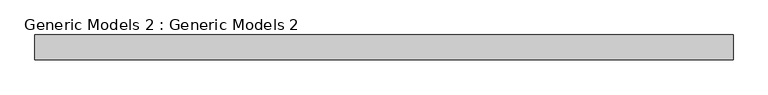
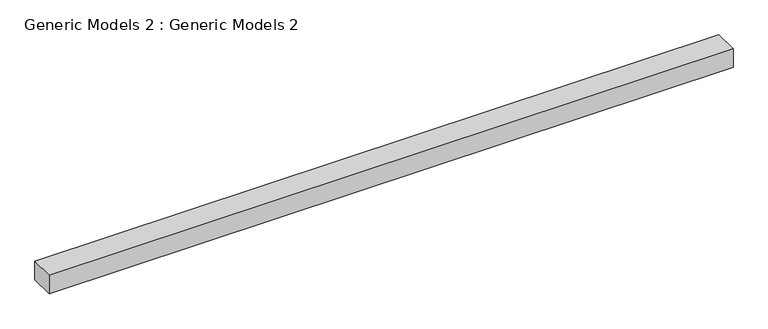
"""IFC4 building model written with IfcOpenShell, lengths in millimetres: proxy geometry, Generic Models 2 : Generic Models 2."""

from ifc_helpers import new_model, si_unit, frame, origin, place, context, project, spatial, polyline, outline, extrude, source, transform, mapped, element, save


def generic_models_2_generic_models_2_383bbf5d(model_context):
    return source(origin(), model_context, "Body", "SweptSolid", [
        extrude(outline(polyline([(-7701.088074, -21405.6128167), (-7701.088074, -21023.5985361), (2966.911926, -21023.5985361), (2966.911926, -21405.6128167), (-7701.088074, -21405.6128167)])), frame((0.0, 0.0, 32832.3835276), z_axis=(0.0, 0.0, 1.0), x_axis=(1.0, 0.0, 0.0)), (0.0, 0.0, 1.0), 304.8),
    ])


if __name__ == "__main__":
    model = new_model("IFC4")
    model_context = context("Model", 3, world=origin())
    ifc_project = project(units=[si_unit("LENGTHUNIT", "METRE", prefix="MILLI")], contexts=[model_context])
    site = spatial("IfcSite", under=ifc_project)
    building = spatial("IfcBuilding", under=site)
    placement = place(None, origin())
    generic_models_2_generic_models_2_shape = generic_models_2_generic_models_2_383bbf5d(model_context)
    element("IfcBuildingElementProxy", 1, Name="Generic Models 2 : Generic Models 2", ObjectType="Generic Models 2 : Generic Models 2", at=placement, inside=building, context=model_context, shape_type="MappedRepresentation", body=[
        mapped(generic_models_2_generic_models_2_shape, transform((0.0, 0.0, 0.0), x_axis=(1.0, 0.0, 0.0), y_axis=(0.0, 1.0, 0.0), z_axis=(0.0, 0.0, 1.0))),
    ])
    save(model, "model.ifc")
